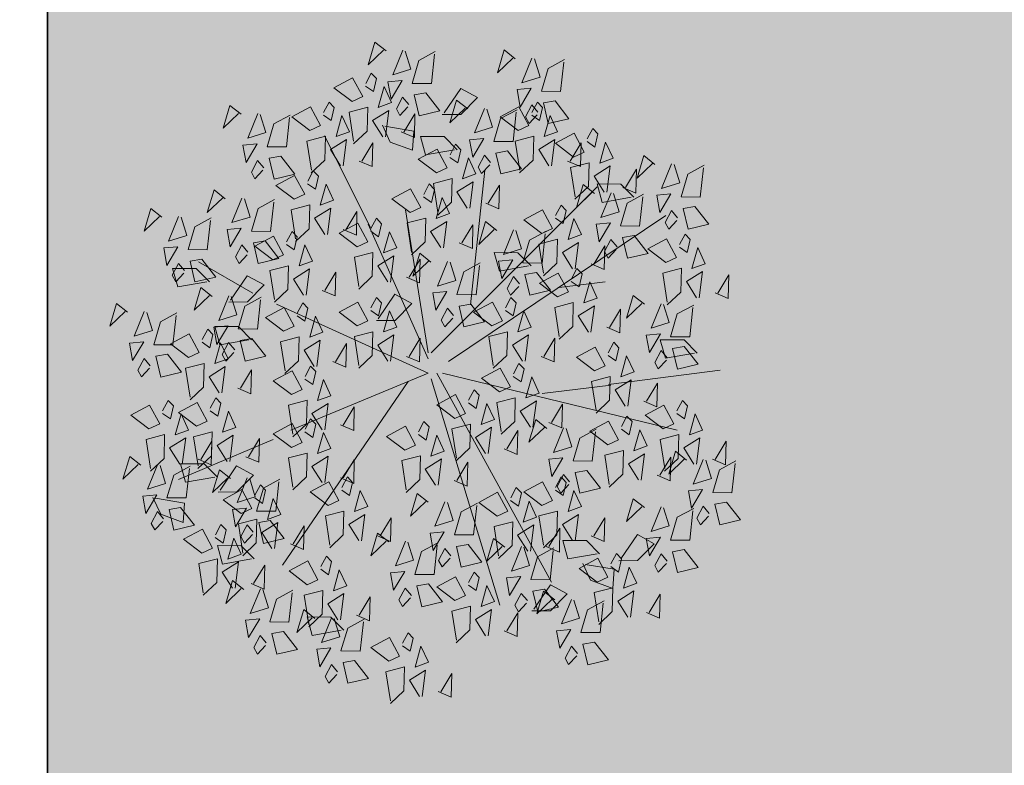
# Model space of a CAD drawing. Units: inches. Extents: x 1704 to 6393, y -157 to 1172.
# Tile 65 of 122: x 1897 to 1937, y 950 to 980. Entities that reach past the tile are written whole.
import ezdxf

# ---------------------------------------------------------------- set-up
doc = ezdxf.new("R2010")
doc.units = ezdxf.units.IN
doc.header["$MEASUREMENT"] = 0
for name, color, linetype, lineweight in [('A-ANNO-DIMS', 7, 'Continuous', 13), ('C-PROP', 7, 'Continuous', 35), ('L-shrub', 74, 'Continuous', 18)]:
    doc.layers.add(name, color=color, linetype=linetype, lineweight=lineweight)
doc.layers.add('L-HRDS-PATT', color=9, linetype='Continuous', lineweight=13, true_color=0xc5c1ba)
doc.styles.get("Standard").update_dxf_attribs({"font": 'arial.ttf'})
doc.dimstyles.get("Standard").update_dxf_attribs({"dimtxt": 6, "dimasz": 2, "dimexe": 0.18, "dimexo": 0.0625, "dimgap": 0.09, "dimtad": 0, "dimtih": 1, "dimtoh": 1, "dimdec": 1, "dimzin": 0, "dimdsep": 46, "dimlunit": 3, "dimtxsty": 'Standard', "dimblk": 'ARCHTICK', "dimcen": 0.09, "dimadec": 0, "dimazin": 0, "dimtfac": 1, "dimtdec": 1, "dimtofl": 0, "dimtmove": 0, "dimatfit": 3, "dimfxl": 1, "dimtolj": 1, "dimtzin": 0, "dimarcsym": 0})

# ---------------------------------------------------------------- blocks, each defined once
blk = doc.blocks.new('flower shrub 2')
at = {"layer": 'L-shrub'}
for p, q in [((-106.23, 211.82), (-92.99, 218)), ((-93.69, 216.06), (-97.6, 193.26)), ((-112.6, 194.32), (-106.23, 211.82)), ((71.95, 198.59), (86.43, 202.67)), ((86.43, 202.67), (86.36, 184.05)), ((-97.6, 193.26), (-112.6, 194.32)), ((-81.12, 192.39), (-66.64, 196.47)), ((-66.64, 196.47), (-66.71, 177.85)), ((75.99, 175.82), (71.95, 198.59)), ((-77.07, 169.62), (-81.12, 192.39)), ((-66.71, 177.85), (-77.08, 167.55)), ((86.36, 184.05), (75.99, 173.75)), ((-145.24, 163.47), (-130.76, 167.54)), ((-141.2, 140.7), (-145.24, 163.47)), ((-130.76, 167.54), (-130.83, 148.93)), ((-88.72, 152.29), (-88.87, 166.9)), ((-87.4, 165.46), (-68.26, 152.47)), ((26.45, 165.53), (40.92, 169.61)), ((30.49, 142.76), (26.45, 165.53)), ((40.92, 169.61), (40.85, 150.99)), ((60.21, 144.02), (60.06, 158.64)), ((61.53, 157.19), (80.67, 144.21)), ((-130.83, 148.93), (-141.21, 138.63)), ((-75.44, 139.25), (-88.72, 152.29)), ((-68.26, 152.47), (-75.44, 139.25)), ((40.85, 150.99), (30.48, 140.69)), ((73.5, 130.99), (60.21, 144.02)), ((80.67, 144.21), (73.5, 130.99)), ((-201.09, 93.22), (-186.61, 97.3)), ((-197.05, 70.45), (-201.09, 93.22)), ((-186.61, 97.3), (-186.68, 78.69)), ((-186.68, 78.69), (-197.06, 68.38)), ((45.73, 28.33), (45.58, 42.95)), ((47.06, 41.5), (66.19, 28.51)), ((179.06, 14.59), (185.43, 32.08)), ((185.43, 32.08), (198.67, 38.26)), ((197.96, 36.32), (194.06, 13.53)), ((59.02, 15.29), (45.73, 28.33)), ((66.19, 28.51), (59.02, 15.29)), ((175.38, 4.39), (189.86, 8.47)), ((194.06, 13.53), (179.06, 14.59)), ((189.86, 8.47), (189.78, -10.15)), ((179.42, -18.38), (175.38, 4.39)), ((189.78, -10.15), (179.41, -20.45)), ((207.07, -23.32), (206.92, -8.7)), ((208.4, -10.15), (227.53, -23.13)), ((227.53, -23.13), (220.36, -36.35)), ((220.36, -36.35), (207.07, -23.32)), ((84.36, -53.46), (98.84, -49.38)), ((88.41, -76.23), (84.36, -53.46)), ((98.84, -49.38), (98.77, -68)), ((98.77, -68), (88.4, -78.3)), ((-181.81, -93.56), (-181.96, -78.94)), ((-180.48, -80.39), (-161.34, -93.38)), ((-168.52, -106.6), (-181.81, -93.56)), ((-161.34, -93.38), (-168.52, -106.6)), ((-141.1, -107.17), (-126.62, -103.09)), ((-137.06, -129.94), (-141.1, -107.17)), ((-126.62, -103.09), (-126.7, -121.71)), ((-157.94, -124.93), (-144.7, -118.75)), ((-145.41, -120.69), (-149.31, -143.48)), ((-126.7, -121.71), (-137.07, -132.01)), ((-164.31, -142.42), (-157.94, -124.93)), ((138.15, -134.03), (152.62, -129.95)), ((152.62, -129.95), (152.55, -148.57)), ((142.19, -156.8), (138.15, -134.03)), ((-149.31, -143.48), (-164.31, -142.42)), ((-142.51, -161.74), (-142.65, -147.12)), ((-141.18, -148.57), (-122.04, -161.55)), ((152.55, -148.57), (142.18, -158.87)), ((-129.22, -174.77), (-142.51, -161.74)), ((-122.04, -161.55), (-129.22, -174.77)), ((16.1, -183.61), (30.58, -179.53)), ((20.14, -206.38), (16.1, -183.61)), ((30.58, -179.53), (30.51, -198.15)), ((30.51, -198.15), (20.14, -208.45))]:
    blk.add_line(p, q, dxfattribs=at)
for points in [[(52.15, 237.83), (59.05, 246.56), (41.2, 251.84), (52.74, 239.81)], [(-67.82, 227.5), (-60.92, 236.23), (-78.77, 241.51), (-67.23, 229.48)], [(-39.32, 221.12), (-28.59, 235.29), (-20.71, 220.61), (-35.41, 212.74), (-39.32, 221.12)], [(29.03, 225.28), (27.99, 236.36), (14.33, 233.94), (29.03, 225.28)], [(52.02, 222.79), (37.77, 218.39), (33.35, 232.62), (52.6, 224.77)], [(-90.95, 214.95), (-91.98, 226.03), (-105.64, 223.61), (-90.95, 214.95)], [(10.23, 220.07), (15.95, 224.84), (6.62, 229.76), (1.48, 226.97), (8.24, 220.66)], [(126.62, 210.97), (133.52, 219.7), (115.67, 224.99), (127.2, 212.95)], [(-109.75, 209.74), (-104.02, 214.51), (-113.35, 219.43), (-118.49, 216.64), (-111.73, 210.33)], [(-67.96, 212.46), (-82.2, 208.06), (-86.62, 222.29), (-67.37, 214.44)], [(-70.39, 219.89), (-47.54, 223.41), (-43.79, 208.84), (-62.4, 209.34), (-72.46, 219.95)], [(49.53, 199.82), (26.54, 202.32), (26.68, 217.36), (44.53, 212.08), (51.52, 199.24)], [(-27.19, 210.46), (-31.5, 204.37), (-21.21, 202.03), (-16.97, 206.05), (-25.13, 210.4)], [(19.2, 206.65), (5.18, 195.71), (1.34, 211.93), (17.57, 215.74), (19.2, 206.65)], [(103.49, 198.43), (102.46, 209.5), (88.8, 207.08), (103.49, 198.43)], [(-100.78, 196.32), (-114.8, 185.38), (-118.63, 201.6), (-102.4, 205.41), (-100.78, 196.32)], [(-70.44, 189.49), (-93.43, 191.99), (-93.29, 207.03), (-75.44, 201.75), (-68.45, 188.91)], [(-66.87, 197.06), (-54.24, 204.99), (-46.3, 192.37), (-66.93, 195)], [(16.53, 190.13), (27.26, 204.31), (35.14, 189.63), (20.44, 181.76), (16.53, 190.13)], [(84.69, 193.22), (90.42, 197.99), (81.09, 202.9), (75.95, 200.11), (82.71, 193.8)], [(126.48, 195.93), (112.24, 191.53), (107.82, 205.76), (127.07, 197.91)], [(-136.54, 179.8), (-125.81, 193.98), (-117.93, 179.3), (-132.63, 171.43), (-136.54, 179.8)], [(-47.57, 123.92), (-79, 197.93)], [(-44.01, 200.58), (-40.16, 190.14), (-27.58, 196), (-44.01, 200.58)], [(-37.25, 183.93), (-26.52, 198.11), (-18.64, 183.43), (-33.34, 175.56), (-37.25, 183.93)], [(-68.32, 182.7), (-45.47, 186.22), (-41.72, 171.65), (-60.33, 172.15), (-70.39, 182.76)], [(-14.54, 188.9), (8.31, 192.42), (12.06, 177.85), (-6.55, 178.35), (-16.61, 188.96)], [(64.56, 171.72), (71.46, 180.45), (53.61, 185.73), (65.15, 173.7)], [(93.66, 179.79), (79.64, 168.86), (75.81, 185.07), (92.04, 188.89), (93.66, 179.79)], [(124, 172.97), (101.01, 175.46), (101.15, 190.5), (119, 185.22), (125.98, 172.38)], [(-167.61, 178.57), (-144.76, 182.09), (-141.01, 167.52), (-159.62, 168.02), (-169.68, 178.63)], [(-63.13, 182.49), (-67.54, 172.28), (-48.93, 171.78), (-63.18, 180.43)], [(28.66, 179.47), (24.35, 173.38), (34.64, 171.04), (38.88, 175.06), (30.72, 179.41)], [(66.94, 139.62), (91.63, 182.23)], [(-78.16, 157.26), (-71.26, 165.99), (-89.12, 171.27), (-77.58, 159.24)], [(-25.12, 173.27), (-29.43, 167.19), (-19.14, 164.84), (-14.9, 168.86), (-23.06, 173.21)], [(-11.02, 166.07), (1.61, 174), (9.54, 161.38), (-11.08, 164.01)], [(41.44, 159.17), (40.4, 170.25), (26.74, 167.83), (41.44, 159.17)], [(141.1, 161.39), (148, 170.12), (130.14, 175.4), (141.68, 163.37)], [(-164.09, 155.74), (-151.46, 163.67), (-143.52, 151.05), (-164.15, 153.68)], [(-124.41, 169.14), (-128.72, 163.05), (-118.43, 160.71), (-114.19, 164.73), (-122.34, 169.08)], [(-105.51, 148.81), (-94.78, 162.99), (-86.9, 148.31), (-101.6, 140.44), (-105.51, 148.81)], [(-64.8, 159.87), (-52.17, 167.8), (-44.24, 155.19), (-64.86, 157.81)], [(-41.95, 163.39), (-38.09, 152.95), (-25.52, 158.81), (-41.95, 163.39)], [(11.84, 169.59), (15.69, 159.15), (28.27, 165.01), (11.84, 169.59)], [(22.64, 153.96), (28.36, 158.73), (19.03, 163.65), (13.89, 160.86), (20.65, 154.55)], [(64.43, 156.68), (50.18, 152.28), (45.76, 166.51), (65.01, 158.66)], [(207.29, 148.99), (214.19, 157.72), (196.34, 163.01), (207.88, 150.97)], [(-165.04, 146.93), (-158.14, 155.66), (-175.99, 160.94), (-164.45, 148.91)], [(-141.23, 159.26), (-137.38, 148.82), (-124.8, 154.68), (-141.23, 159.26)], [(-101.29, 144.71), (-102.33, 155.79), (-115.98, 153.37), (-101.29, 144.71)], [(117.97, 148.84), (116.93, 159.92), (103.28, 157.5), (117.97, 148.84)], [(140.96, 146.35), (126.72, 141.95), (122.3, 156.18), (141.55, 148.33)], [(-136.58, 147.58), (-113.73, 151.1), (-109.98, 136.53), (-128.59, 137.03), (-138.65, 147.64)], [(-120.09, 139.5), (-114.36, 144.27), (-123.69, 149.19), (-128.83, 146.4), (-122.07, 140.09)], [(-78.3, 142.22), (-92.54, 137.81), (-96.96, 152.05), (-77.71, 144.2)], [(-7.28, 151.5), (-11.69, 141.29), (6.92, 140.79), (-7.33, 149.44)], [(31.61, 140.54), (17.59, 129.6), (13.76, 145.82), (29.99, 149.63), (31.61, 140.54)], [(61.95, 133.71), (38.95, 136.21), (39.09, 151.25), (56.94, 145.97), (63.93, 133.13)], [(99.17, 143.63), (104.9, 148.4), (95.57, 153.32), (90.43, 150.53), (97.19, 144.22)], [(184.16, 136.45), (183.13, 147.53), (169.47, 145.1), (184.16, 136.45)], [(-188.17, 134.38), (-189.2, 145.46), (-202.86, 143.04), (-188.17, 134.38)], [(-165.18, 131.89), (-179.42, 127.48), (-183.84, 141.72), (-164.59, 133.87)], [(-160.34, 141.17), (-164.76, 130.96), (-146.15, 130.46), (-160.4, 139.11)], [(-61.06, 145.31), (-65.47, 135.09), (-46.86, 134.59), (-61.11, 143.24)], [(108.14, 130.21), (94.12, 119.27), (90.29, 135.49), (106.52, 139.3), (108.14, 130.21)], [(138.48, 123.38), (115.49, 125.88), (115.63, 140.92), (133.48, 135.64), (140.46, 122.8)], [(165.36, 131.24), (171.09, 136.01), (161.76, 140.92), (156.62, 138.13), (163.38, 131.82)], [(207.15, 133.95), (192.91, 129.55), (188.49, 143.78), (207.74, 135.93)], [(-206.97, 129.17), (-201.24, 133.94), (-210.57, 138.86), (-215.71, 136.07), (-208.95, 129.76)], [(-133.06, 124.75), (-120.43, 132.68), (-112.5, 120.06), (-133.12, 122.69)], [(-111.12, 126.07), (-125.14, 115.14), (-128.97, 131.36), (-112.74, 135.17), (-111.12, 126.07)], [(-80.78, 119.25), (-103.77, 121.75), (-103.63, 136.79), (-85.78, 131.5), (-78.8, 118.66)], [(-93.39, 138.15), (-97.69, 132.06), (-87.4, 129.72), (-83.16, 133.74), (-91.32, 138.09)], [(93.06, 124.02), (103.79, 138.2), (111.67, 123.52), (96.98, 115.65), (93.06, 124.02)], [(-198, 115.75), (-212.02, 104.81), (-215.85, 121.03), (-199.62, 124.84), (-198, 115.75)], [(-167.66, 108.92), (-190.65, 111.42), (-190.51, 126.46), (-172.66, 121.17), (-165.67, 108.33)], [(-110.21, 128.27), (-106.35, 117.83), (-93.78, 123.69), (-110.21, 128.27)], [(-53.8, 109.56), (-43.07, 123.73), (-35.19, 109.05), (-49.89, 101.18), (-53.8, 109.56)], [(-12.43, 109.56), (-1.7, 123.73), (6.18, 109.05), (-8.52, 101.18), (-12.43, 109.56)], [(37.21, 115.75), (47.94, 129.93), (55.82, 115.25), (41.13, 107.38), (37.21, 115.75)], [(61.99, 122.79), (84.85, 126.31), (88.59, 111.74), (69.98, 112.24), (59.92, 122.85)], [(174.33, 117.81), (160.31, 106.88), (156.48, 123.09), (172.71, 126.91), (174.33, 117.81)], [(204.67, 110.99), (181.68, 113.48), (181.82, 128.52), (199.67, 123.24), (206.65, 110.4)], [(-2.25, 17.94), (-145.94, 116.61)], [(6.14, 114.53), (29, 118.04), (32.74, 103.47), (14.13, 103.98), (4.07, 114.58)], [(4.49, 2.24), (58.38, 121.09)], [(140.64, 107.49), (151.37, 121.67), (159.25, 106.99), (144.55, 99.12), (140.64, 107.49)], [(-161.36, 97.16), (-150.63, 111.34), (-142.75, 96.66), (-157.45, 88.79), (-161.36, 97.16)], [(-129.32, 110.18), (-133.73, 99.97), (-115.12, 99.47), (-129.37, 108.12)], [(-84.87, 108.33), (-62.02, 111.85), (-58.27, 97.28), (-76.88, 97.78), (-86.94, 108.38)], [(-43.5, 108.33), (-20.65, 111.85), (-16.9, 97.28), (-35.51, 97.78), (-45.57, 108.38)], [(4.49, 2.24), (-40.41, 109.88)], [(105.19, 113.36), (100.89, 107.27), (111.17, 104.93), (115.42, 108.95), (107.26, 113.3)], [(109.57, 106.26), (132.42, 109.78), (136.17, 95.21), (117.56, 95.71), (107.5, 106.32)], [(194.42, 95.09), (205.15, 109.27), (213.03, 94.59), (198.33, 86.72), (194.42, 95.09)], [(-187.79, 91.15), (-180.89, 99.88), (-198.75, 105.16), (-187.21, 93.13)], [(49.34, 105.09), (45.04, 99.01), (55.32, 96.67), (59.57, 100.68), (51.41, 105.04)], [(65.51, 99.96), (78.14, 107.89), (86.08, 95.27), (65.46, 97.9)], [(88.37, 103.48), (92.23, 93.04), (104.8, 98.9), (88.37, 103.48)], [(-192.43, 95.93), (-169.58, 99.45), (-165.83, 84.88), (-184.44, 85.38), (-194.5, 95.99)], [(-99.31, 80.63), (-88.58, 94.81), (-80.7, 80.13), (-95.39, 72.26), (-99.31, 80.63)], [(-81.35, 85.5), (-68.72, 93.43), (-60.78, 80.81), (-81.41, 83.43)], [(-41.67, 98.9), (-45.98, 92.81), (-35.69, 90.47), (-31.45, 94.49), (-39.6, 98.84)], [(-39.98, 85.5), (-27.35, 93.43), (-19.41, 80.81), (-40.04, 83.43)], [(-0.3, 98.9), (-4.61, 92.81), (5.68, 90.47), (9.92, 94.49), (1.76, 98.84)], [(9.66, 91.7), (22.29, 99.62), (30.23, 87.01), (9.61, 89.63)], [(32.52, 95.21), (36.38, 84.78), (48.95, 90.64), (32.52, 95.21)], [(152.77, 96.83), (148.46, 90.75), (158.75, 88.4), (162.99, 92.42), (154.83, 96.77)], [(163.35, 93.87), (186.2, 97.38), (189.95, 82.82), (171.34, 83.32), (161.28, 93.92)], [(-210.92, 78.6), (-211.96, 89.68), (-225.62, 87.26), (-210.92, 78.6)], [(-187.93, 76.11), (-202.17, 71.7), (-206.59, 85.94), (-187.34, 78.09)], [(-149.23, 86.5), (-153.54, 80.42), (-143.25, 78.07), (-139.01, 82.09), (-147.17, 86.44)], [(-58.49, 89.02), (-54.64, 78.58), (-42.06, 84.44), (-58.49, 89.02)], [(-17.12, 89.02), (-13.27, 78.58), (-0.69, 84.44), (-17.12, 89.02)], [(69.26, 85.39), (64.84, 75.18), (83.45, 74.68), (69.2, 83.33)], [(113.09, 83.43), (125.72, 91.36), (133.65, 78.75), (113.03, 81.37)], [(135.94, 86.95), (139.8, 76.51), (152.38, 82.37), (135.94, 86.95)], [(-229.72, 73.39), (-223.99, 78.16), (-233.32, 83.08), (-238.46, 80.29), (-231.7, 73.98)], [(-188.91, 73.1), (-176.28, 81.03), (-168.35, 68.42), (-188.97, 71.04)], [(-130.38, 79.41), (-107.52, 82.92), (-103.78, 68.35), (-122.39, 68.86), (-132.45, 79.46)], [(118.58, 47.68), (190.43, 83.56)], [(166.87, 71.04), (179.5, 78.96), (187.44, 66.35), (166.81, 68.97)], [(206.55, 84.43), (202.24, 78.35), (212.53, 76.01), (216.77, 80.02), (208.61, 84.38)], [(-190.41, 53.14), (-213.4, 55.64), (-213.26, 70.68), (-195.41, 65.39), (-188.43, 52.55)], [(-166.05, 76.62), (-162.2, 66.18), (-149.62, 72.04), (-166.05, 76.62)], [(-87.18, 69.97), (-91.48, 63.89), (-81.2, 61.54), (-76.95, 65.56), (-85.11, 69.92)], [(-77.6, 70.93), (-82.02, 60.72), (-63.41, 60.22), (-77.66, 68.87)], [(-36.23, 70.93), (-40.65, 60.72), (-22.04, 60.22), (-36.29, 68.87)], [(13.41, 77.13), (8.99, 66.92), (27.6, 66.41), (13.35, 75.06)], [(41.35, 57.91), (52.08, 72.09), (59.96, 57.41), (45.26, 49.54), (41.35, 57.91)], [(103.41, 57.91), (114.13, 72.09), (122.01, 57.41), (107.32, 49.54), (103.41, 57.91)], [(189.73, 74.55), (193.58, 64.12), (206.16, 69.98), (189.73, 74.55)], [(217.17, 62.04), (227.9, 76.22), (235.78, 61.54), (221.08, 53.67), (217.17, 62.04)], [(-220.75, 59.96), (-234.77, 49.03), (-238.6, 65.25), (-222.37, 69.06), (-220.75, 59.96)], [(-126.86, 56.58), (-114.23, 64.5), (-106.29, 51.89), (-126.91, 54.51)], [(116.83, 68.87), (112.42, 58.65), (131.03, 58.15), (116.78, 66.8)], [(186.1, 60.81), (208.96, 64.33), (212.7, 49.76), (194.09, 50.26), (184.03, 60.87)], [(-185.17, 58.54), (-189.58, 48.32), (-170.97, 47.82), (-185.22, 56.47)], [(-104, 60.09), (-100.14, 49.66), (-87.57, 55.52), (-104, 60.09)], [(10.28, 56.68), (33.14, 60.2), (36.88, 45.63), (18.27, 46.13), (8.21, 56.74)], [(72.33, 56.68), (95.19, 60.2), (98.94, 45.63), (80.33, 46.13), (70.27, 56.74)], [(170.61, 56.47), (166.2, 46.26), (184.81, 45.75), (170.56, 54.41)], [(-221.35, 33.12), (-210.62, 47.29), (-202.74, 32.61), (-217.44, 24.74), (-221.35, 33.12)], [(-127.81, 33.3), (-120.91, 42.03), (-138.76, 47.31), (-127.22, 35.28)], [(15.72, 2.24), (121.24, 49.33)], [(53.48, 47.25), (49.18, 41.16), (59.46, 38.82), (63.71, 42.84), (55.55, 47.19)], [(115.53, 47.25), (111.23, 41.16), (121.51, 38.82), (125.76, 42.84), (117.6, 47.19)], [(229.3, 51.38), (225, 45.3), (235.28, 42.95), (239.53, 46.97), (231.37, 51.32)], [(256.93, 35.37), (263.83, 44.1), (245.98, 49.38), (257.52, 37.35)], [(-123.11, 42.01), (-127.53, 31.79), (-108.92, 31.29), (-123.17, 39.94)], [(13.8, 33.85), (26.43, 41.78), (34.37, 29.16), (13.74, 31.79)], [(75.86, 33.85), (88.48, 41.78), (96.42, 29.16), (75.8, 31.79)], [(189.62, 37.98), (202.25, 45.91), (210.19, 33.29), (189.57, 35.92)], [(212.48, 41.5), (216.34, 31.06), (228.91, 36.92), (212.48, 41.5)], [(-252.42, 31.89), (-229.56, 35.41), (-225.82, 20.84), (-244.43, 21.34), (-254.49, 31.94)], [(-150.93, 20.75), (-151.97, 31.83), (-165.63, 29.41), (-150.93, 20.75)], [(-55.87, 20.72), (-45.14, 34.9), (-37.26, 20.22), (-51.96, 12.35), (-55.87, 20.72)], [(36.66, 37.37), (40.51, 26.93), (53.09, 32.79), (36.66, 37.37)], [(98.71, 37.37), (102.57, 26.93), (115.14, 32.79), (98.71, 37.37)], [(233.81, 22.82), (232.77, 33.9), (219.11, 31.48), (233.81, 22.82)], [(-169.73, 15.55), (-164.01, 20.31), (-173.34, 25.23), (-178.48, 22.44), (-171.72, 16.13)], [(-127.94, 18.26), (-142.19, 13.86), (-146.61, 28.09), (-127.36, 20.24)], [(130.3, 16.59), (141.02, 30.77), (148.91, 16.09), (134.21, 8.22), (130.3, 16.59)], [(193.37, 23.42), (188.95, 13.2), (207.56, 12.7), (193.31, 21.35)], [(215.01, 17.61), (220.73, 22.38), (211.4, 27.3), (206.26, 24.51), (213.02, 18.2)], [(256.8, 20.33), (242.55, 15.92), (238.13, 30.16), (257.38, 22.31)], [(-248.9, 9.06), (-236.27, 16.99), (-228.33, 4.37), (-248.95, 7)], [(-209.22, 22.46), (-213.52, 16.37), (-203.24, 14.03), (-198.99, 18.05), (-207.15, 22.4)], [(-96.78, 2.31), (-89.88, 11.04), (-107.73, 16.33), (-96.19, 4.29)], [(-86.94, 19.49), (-64.08, 23.01), (-60.34, 8.44), (-78.95, 8.94), (-89.01, 19.55)], [(17.55, 19.28), (13.13, 9.07), (31.74, 8.57), (17.49, 17.22)], [(20.21, 2.24), (132.47, 20.18)], [(79.6, 19.28), (75.19, 9.07), (93.8, 8.57), (79.54, 17.22)], [(99.22, 15.36), (122.08, 18.88), (125.83, 4.31), (107.22, 4.81), (97.16, 15.42)], [(-226.04, 12.58), (-222.18, 2.14), (-209.61, 8), (-226.04, 12.58)], [(-160.76, 2.12), (-174.78, -8.81), (-178.61, 7.4), (-162.38, 11.22), (-160.76, 2.12)], [(-130.42, -4.7), (-153.42, -2.21), (-153.28, 12.83), (-135.43, 7.55), (-128.44, -5.29)], [(-43.74, 10.06), (-48.04, 3.98), (-37.76, 1.63), (-33.51, 5.65), (-41.67, 10)], [(91.45, 0.25), (98.35, 8.98), (80.5, 14.26), (92.04, 2.23)], [(161.32, -4.07), (172.05, 10.11), (179.93, -4.57), (165.24, -12.44), (161.32, -4.07)], [(223.98, 4.18), (209.96, -6.75), (206.13, 9.47), (222.35, 13.28), (223.98, 4.18)], [(254.32, -2.64), (231.32, -0.14), (231.46, 14.9), (249.31, 9.61), (256.3, -3.23)], [(0, 0), (-177.37, -53.82)], [(-119.91, -10.23), (-120.94, 0.84), (-134.6, -1.58), (-119.91, -10.23)], [(-83.42, -3.34), (-70.79, 4.59), (-62.85, -8.02), (-83.47, -5.4)], [(-60.56, 0.18), (-56.71, -10.26), (-44.13, -4.4), (-60.56, 0.18)], [(20.21, 0), (150.43, -130.06)], [(102.75, -7.47), (115.38, 0.46), (123.31, -12.16), (102.69, -9.53)], [(142.42, 5.93), (138.12, -0.16), (148.4, -2.5), (152.65, 1.52), (144.49, 5.87)], [(-245.15, -5.51), (-249.57, -15.72), (-230.96, -16.22), (-245.21, -7.57)], [(-173.77, -18.53), (-163.04, -4.35), (-155.16, -19.03), (-169.86, -26.9), (-173.77, -18.53)], [(4.49, -4.48), (-159.41, -94.18)], [(-138.71, -15.44), (-132.98, -10.67), (-142.31, -5.76), (-147.45, -8.55), (-140.69, -14.86)], [(-96.92, -12.73), (-111.16, -17.13), (-115.58, -2.9), (-96.33, -10.75)], [(-31.05, -18.53), (-20.32, -4.35), (-12.44, -19.03), (-27.13, -26.9), (-31.05, -18.53)], [(68.33, -12.3), (67.29, -1.22), (53.63, -3.64), (68.33, -12.3)], [(91.32, -14.79), (77.07, -19.2), (72.66, -4.96), (91.9, -12.81)], [(125.6, -3.95), (129.46, -14.39), (142.03, -8.53), (125.6, -3.95)], [(130.25, -5.3), (153.11, -1.78), (156.85, -16.35), (138.24, -15.85), (128.18, -5.24)], [(4.49, -8.97), (-40.41, -192.85)], [(13.47, -13.45), (127.98, -183.88)], [(49.53, -17.51), (55.25, -12.74), (45.92, -7.82), (40.78, -10.61), (47.54, -16.92)], [(173.45, -14.73), (169.15, -20.81), (179.43, -23.16), (183.68, -19.14), (175.52, -14.79)], [(211.43, -28.68), (218.32, -19.95), (200.47, -14.66), (212.01, -26.7)], [(-204.84, -19.76), (-181.99, -16.24), (-178.24, -30.81), (-196.85, -30.31), (-206.91, -19.7)], [(-129.74, -28.87), (-143.76, -39.8), (-147.59, -23.59), (-131.36, -19.77), (-129.74, -28.87)], [(-99.4, -35.69), (-122.39, -33.2), (-122.25, -18.16), (-104.4, -23.44), (-97.41, -36.28)], [(-79.67, -17.9), (-84.09, -28.12), (-65.48, -28.62), (-79.73, -19.97)], [(-62.12, -19.76), (-39.26, -16.24), (-35.52, -30.81), (-54.13, -30.31), (-64.19, -19.7)], [(58.5, -30.94), (44.48, -41.87), (40.65, -25.65), (56.88, -21.84), (58.5, -30.94)], [(88.84, -37.76), (65.84, -35.27), (65.98, -20.22), (83.83, -25.51), (90.82, -38.35)], [(106.49, -22.04), (102.08, -32.25), (120.69, -32.75), (106.44, -24.1)], [(133.77, -28.13), (146.4, -20.2), (154.34, -32.82), (133.72, -30.19)], [(-161.65, -29.19), (-165.95, -35.28), (-155.67, -37.62), (-151.42, -33.6), (-159.58, -29.25)], [(-18.92, -29.19), (-23.22, -35.28), (-12.94, -37.62), (-8.69, -33.6), (-16.85, -29.25)], [(57.96, -30.81), (163.48, -42.02)], [(156.63, -24.61), (160.49, -35.05), (173.06, -29.19), (156.63, -24.61)], [(188.3, -41.22), (187.26, -30.14), (173.6, -32.57), (188.3, -41.22)], [(-201.32, -42.59), (-188.69, -34.66), (-180.76, -47.28), (-201.38, -44.65)], [(-107.58, -51.59), (-96.85, -37.41), (-88.97, -52.09), (-103.67, -59.96), (-107.58, -51.59)], [(-58.6, -42.59), (-45.97, -34.66), (-38.03, -47.28), (-58.65, -44.65)], [(41.35, -47.45), (52.08, -33.28), (59.96, -47.96), (45.26, -55.83), (41.35, -47.45)], [(116.28, -51.4), (123.17, -42.67), (105.32, -37.39), (116.86, -49.42)], [(169.5, -46.43), (175.23, -41.66), (165.89, -36.75), (160.76, -39.54), (167.52, -45.85)], [(211.29, -43.72), (197.04, -48.12), (192.63, -33.89), (211.88, -41.74)], [(-178.47, -39.07), (-174.61, -49.51), (-162.04, -43.65), (-178.47, -39.07)], [(-131.94, -57.6), (-125.04, -48.87), (-142.9, -43.59), (-131.36, -55.62)], [(-35.74, -39.07), (-31.88, -49.51), (-19.31, -43.65), (-35.74, -39.07)], [(-10.36, -53.65), (0.37, -39.48), (8.25, -54.15), (-6.45, -62.02), (-10.36, -53.65)], [(10.28, -48.68), (33.14, -45.17), (36.88, -59.73), (18.27, -59.23), (8.21, -48.63)], [(137.52, -42.69), (133.1, -52.91), (151.71, -53.41), (137.46, -44.76)], [(-138.65, -52.81), (-115.8, -49.3), (-112.05, -63.87), (-130.66, -63.36), (-140.72, -52.76)], [(-41.43, -54.88), (-18.58, -51.36), (-14.83, -65.93), (-33.44, -65.43), (-43.5, -54.82)], [(93.15, -63.95), (92.11, -52.87), (78.45, -55.29), (93.15, -63.95)], [(178.47, -59.86), (164.45, -70.79), (160.62, -54.58), (176.85, -50.76), (178.47, -59.86)], [(208.81, -66.68), (185.82, -64.19), (185.95, -49.15), (203.81, -54.43), (210.79, -67.27)], [(194.42, -68.11), (205.15, -53.94), (213.03, -68.62), (198.33, -76.49), (194.42, -68.11)], [(250.73, -65.86), (257.63, -57.13), (239.78, -51.85), (251.31, -63.88)], [(-197.58, -57.16), (-201.99, -67.37), (-183.38, -67.87), (-197.63, -59.22)], [(-155.07, -70.15), (-156.11, -59.07), (-169.77, -61.49), (-155.07, -70.15)], [(-54.85, -57.16), (-59.27, -67.37), (-40.66, -67.87), (-54.91, -59.22)], [(53.48, -58.12), (49.18, -64.2), (59.46, -66.54), (63.71, -62.52), (55.55, -58.17)], [(74.35, -69.16), (80.08, -64.39), (70.74, -59.47), (65.6, -62.26), (72.37, -68.57)], [(116.14, -66.44), (101.89, -70.85), (97.48, -56.61), (116.73, -64.46)], [(-173.87, -75.36), (-168.14, -70.59), (-177.47, -65.67), (-182.61, -68.46), (-175.85, -74.77)], [(-132.08, -72.64), (-146.33, -77.04), (-150.74, -62.81), (-131.49, -70.66)], [(-135.13, -75.64), (-122.5, -67.72), (-114.56, -80.33), (-135.19, -77.71)], [(-95.45, -62.25), (-99.76, -68.33), (-89.47, -70.68), (-85.23, -66.66), (-93.39, -62.3)], [(1.77, -64.31), (-2.54, -70.4), (7.75, -72.74), (11.99, -68.72), (3.83, -64.37)], [(13.8, -71.51), (26.43, -63.59), (34.37, -76.2), (13.74, -73.58)], [(36.66, -67.99), (40.51, -78.43), (53.09, -72.57), (36.66, -67.99)], [(163.35, -69.34), (186.2, -65.83), (189.95, -80.39), (171.34, -79.89), (161.28, -69.29)], [(227.6, -78.41), (226.56, -67.33), (212.91, -69.75), (227.6, -78.41)], [(-112.27, -72.13), (-108.42, -82.56), (-95.84, -76.7), (-112.27, -72.13)], [(-99.31, -86.71), (-88.58, -72.53), (-80.7, -87.21), (-95.39, -95.08), (-99.31, -86.71)], [(-38.86, -90.66), (-31.96, -81.92), (-49.81, -76.64), (-38.27, -88.67)], [(-37.91, -77.71), (-25.28, -69.78), (-17.35, -82.4), (-37.97, -79.77)], [(-15.06, -74.19), (-11.2, -84.63), (1.38, -78.77), (-15.06, -74.19)], [(83.32, -82.58), (69.3, -93.52), (65.47, -77.3), (81.7, -73.49), (83.32, -82.58)], [(113.66, -89.41), (90.67, -86.91), (90.8, -71.87), (108.65, -77.16), (115.64, -90)], [(113.75, -86.71), (124.48, -72.53), (132.36, -87.21), (117.66, -95.08), (113.75, -86.71)], [(208.8, -83.62), (214.53, -78.85), (205.2, -73.93), (200.06, -76.72), (206.82, -83.03)], [(250.59, -80.9), (236.35, -85.31), (231.93, -71.07), (251.18, -78.92)], [(-173.31, -96.85), (-166.41, -88.12), (-184.27, -82.84), (-172.73, -94.87)], [(-164.9, -88.78), (-178.92, -99.72), (-182.75, -83.5), (-166.52, -79.68), (-164.9, -88.78)], [(-134.56, -95.61), (-157.55, -93.11), (-157.42, -78.07), (-139.56, -83.35), (-132.58, -96.19)], [(-130.38, -87.94), (-107.52, -84.42), (-103.78, -98.99), (-122.39, -98.48), (-132.45, -87.88)], [(82.68, -87.94), (105.53, -84.42), (109.28, -98.99), (90.67, -98.48), (80.61, -87.88)], [(166.87, -92.17), (179.5, -84.24), (187.44, -96.86), (166.81, -94.24)], [(206.55, -78.77), (202.24, -84.86), (212.53, -87.2), (216.77, -83.18), (208.61, -78.83)], [(-131.39, -90.21), (-135.8, -100.43), (-117.19, -100.93), (-131.44, -92.28)], [(-61.99, -103.2), (-63.02, -92.12), (-76.68, -94.54), (-61.99, -103.2)], [(-34.17, -92.28), (-38.58, -102.49), (-19.97, -102.99), (-34.22, -94.34)], [(-4.91, -140.69), (-11.65, -86.87)], [(17.55, -86.08), (13.13, -96.29), (31.74, -96.8), (17.49, -88.14)], [(64.1, -99.1), (74.83, -84.93), (82.71, -99.61), (68.02, -107.48), (64.1, -99.1)], [(189.73, -88.65), (193.58, -99.09), (206.16, -93.23), (189.73, -88.65)], [(217.77, -97.05), (203.75, -107.98), (199.92, -91.76), (216.15, -87.95), (217.77, -97.05)], [(248.11, -103.87), (225.12, -101.38), (225.26, -86.33), (243.11, -91.62), (250.09, -104.46)], [(-196.44, -109.4), (-197.48, -98.32), (-211.14, -100.74), (-196.44, -109.4)], [(-87.18, -97.37), (-91.48, -103.45), (-81.2, -105.8), (-76.95, -101.78), (-85.11, -97.42)], [(-80.79, -108.41), (-75.06, -103.64), (-84.39, -98.73), (-89.53, -101.51), (-82.77, -107.82)], [(-39, -105.7), (-53.24, -110.1), (-57.66, -95.86), (-38.41, -103.72)], [(33.03, -100.33), (55.89, -96.81), (59.63, -111.38), (41.02, -110.88), (30.96, -100.28)], [(125.88, -97.37), (121.57, -103.45), (131.86, -105.8), (136.1, -101.78), (127.94, -97.42)], [(173.73, -111.5), (184.46, -97.32), (192.34, -112), (177.65, -119.87), (173.73, -111.5)], [(-215.24, -114.61), (-209.51, -109.84), (-218.84, -104.92), (-223.98, -107.71), (-217.22, -114.02)], [(-173.45, -111.89), (-187.7, -116.3), (-192.11, -102.06), (-172.86, -109.91)], [(-126.86, -110.76), (-114.23, -102.84), (-106.29, -115.45), (-126.91, -112.83)], [(-104, -107.25), (-100.14, -117.69), (-87.57, -111.82), (-104, -107.25)], [(71.43, -100.32), (75.92, -136.2)], [(86.2, -110.76), (98.83, -102.84), (106.76, -115.45), (86.14, -112.83)], [(109.05, -107.25), (112.91, -117.69), (125.48, -111.82), (109.05, -107.25)], [(170.61, -106.74), (166.2, -116.95), (184.81, -117.46), (170.56, -108.8)], [(-71.82, -121.84), (-85.84, -132.77), (-89.67, -116.56), (-73.44, -112.74), (-71.82, -121.84)], [(-41.48, -128.66), (-64.47, -126.17), (-64.33, -111.13), (-46.48, -116.41), (-39.5, -129.25)], [(6.19, -128.03), (16.91, -113.85), (24.8, -128.53), (10.1, -136.4), (6.19, -128.03)], [(36.55, -123.16), (49.18, -115.23), (57.12, -127.85), (36.5, -125.22)], [(76.23, -109.76), (71.93, -115.85), (82.21, -118.19), (86.46, -114.17), (78.3, -109.82)], [(145.23, -127.84), (152.13, -119.11), (134.28, -113.83), (145.82, -125.86)], [(142.66, -112.73), (165.52, -109.21), (169.26, -123.78), (150.65, -123.28), (140.59, -112.67)], [(-206.27, -128.04), (-220.29, -138.97), (-224.12, -122.75), (-207.89, -118.94), (-206.27, -128.04)], [(-175.93, -134.86), (-198.92, -132.36), (-198.79, -117.32), (-180.93, -122.61), (-173.95, -135.45)], [(-159.29, -130.09), (-148.56, -115.91), (-140.68, -130.59), (-155.38, -138.46), (-159.29, -130.09)], [(59.41, -119.64), (63.27, -130.08), (75.84, -124.22), (59.41, -119.64)], [(185.86, -122.16), (181.56, -128.24), (191.84, -130.59), (196.09, -126.57), (187.93, -122.22)], [(-190.37, -131.32), (-167.51, -127.8), (-163.76, -142.37), (-182.37, -141.87), (-192.43, -131.26)], [(-123.11, -125.33), (-127.53, -135.55), (-108.92, -136.05), (-123.17, -127.4)], [(-51.73, -138.36), (-41, -124.18), (-33.12, -138.86), (-47.82, -146.73), (-51.73, -138.36)], [(-24.89, -129.25), (-2.03, -125.74), (1.72, -140.31), (-16.89, -139.8), (-26.95, -129.2)], [(89.94, -125.33), (85.53, -135.55), (104.14, -136.05), (89.89, -127.4)], [(122.11, -140.39), (121.07, -129.31), (107.41, -131.73), (122.11, -140.39)], [(146.18, -135.56), (158.81, -127.63), (166.75, -140.24), (146.13, -137.62)], [(-82.8, -139.58), (-59.95, -136.07), (-56.2, -150.64), (-74.81, -150.13), (-84.87, -139.53)], [(18.31, -138.69), (14.01, -144.77), (24.29, -147.12), (28.54, -143.1), (20.38, -138.74)], [(40.3, -137.73), (35.89, -147.94), (54.49, -148.44), (40.24, -139.79)], [(103.31, -145.6), (109.03, -140.83), (99.7, -135.91), (94.56, -138.7), (101.33, -145.01)], [(145.1, -142.88), (130.85, -147.29), (126.44, -133.05), (145.68, -140.9)], [(169.04, -132.04), (172.9, -142.48), (185.47, -136.62), (169.04, -132.04)], [(-186.84, -154.15), (-174.21, -146.22), (-166.28, -158.84), (-186.9, -156.21)], [(-147.17, -140.75), (-151.47, -146.84), (-141.19, -149.18), (-136.94, -145.16), (-145.1, -140.81)], [(-21.36, -152.08), (-8.73, -144.16), (-0.8, -156.77), (-21.42, -154.15)], [(-4.49, -139.03), (6.74, -226.49)], [(-163.99, -150.63), (-160.13, -161.07), (-147.56, -155.21), (-163.99, -150.63)], [(-100.92, -167.09), (-94.02, -158.36), (-111.87, -153.08), (-100.33, -165.11)], [(-39.6, -149.02), (-43.91, -155.1), (-33.62, -157.44), (-29.38, -153.43), (-37.54, -149.07)], [(1.49, -148.57), (5.35, -159), (17.92, -153.14), (1.49, -148.57)], [(58.36, -167.09), (65.26, -158.36), (47.41, -153.08), (58.94, -165.11)], [(112.28, -159.02), (98.26, -169.96), (94.43, -153.74), (110.66, -149.93), (112.28, -159.02)], [(142.62, -165.85), (119.63, -163.35), (119.76, -148.31), (137.61, -153.6), (144.6, -166.44)], [(149.93, -150.12), (145.52, -160.34), (164.12, -160.84), (149.87, -152.19)], [(-79.28, -162.41), (-66.65, -154.49), (-58.72, -167.1), (-79.34, -164.48)], [(-56.42, -158.9), (-52.57, -169.33), (-39.99, -163.47), (-56.42, -158.9)], [(167.99, -175.36), (174.89, -166.63), (157.04, -161.34), (168.57, -173.38)], [(-183.1, -168.72), (-187.51, -178.93), (-168.9, -179.43), (-183.15, -170.78)], [(-124.04, -179.64), (-125.08, -168.56), (-138.74, -170.98), (-124.04, -179.64)], [(-39.32, -181.74), (-28.59, -167.56), (-20.71, -182.24), (-35.41, -190.11), (-39.32, -181.74)], [(-17.62, -166.65), (-22.03, -176.87), (-3.42, -177.37), (-17.67, -168.72)], [(35.23, -179.64), (34.2, -168.56), (20.54, -170.98), (35.23, -179.64)], [(90.99, -183.81), (101.72, -169.63), (109.6, -184.31), (94.91, -192.18), (90.99, -183.81)], [(-142.84, -184.85), (-137.12, -180.08), (-146.45, -175.17), (-151.59, -177.95), (-144.83, -184.26)], [(-101.05, -182.14), (-115.3, -186.54), (-119.71, -172.3), (-100.47, -180.15)], [(-75.54, -176.98), (-79.95, -187.19), (-61.34, -187.7), (-75.59, -179.05)], [(16.43, -184.85), (22.16, -180.08), (12.83, -175.17), (7.69, -177.95), (14.45, -184.26)], [(58.22, -182.14), (43.98, -186.54), (39.56, -172.3), (58.81, -180.15)], [(144.86, -187.9), (143.83, -176.83), (130.17, -179.25), (144.86, -187.9)], [(-70.39, -182.97), (-47.54, -179.45), (-43.79, -194.02), (-62.4, -193.52), (-72.46, -182.91)], [(59.92, -185.03), (82.78, -181.52), (86.52, -196.09), (67.91, -195.58), (57.85, -184.98)], [(126.06, -193.11), (131.79, -188.35), (122.46, -183.43), (117.32, -186.22), (124.08, -192.53)], [(167.85, -190.4), (153.61, -194.8), (149.19, -180.57), (168.44, -188.42)], [(-133.87, -198.28), (-147.89, -209.21), (-151.72, -192.99), (-135.49, -189.18), (-133.87, -198.28)], [(-103.53, -205.1), (-126.52, -202.61), (-126.39, -187.57), (-108.54, -192.85), (-101.55, -205.69)], [(-63.68, -200.15), (-56.78, -191.42), (-74.64, -186.14), (-63.1, -198.17)], [(-27.19, -192.4), (-31.5, -198.49), (-21.21, -200.83), (-16.97, -196.81), (-25.13, -192.46)], [(25.4, -198.28), (11.38, -209.21), (7.55, -192.99), (23.78, -189.18), (25.4, -198.28)], [(55.74, -205.1), (32.75, -202.61), (32.89, -187.57), (50.74, -192.85), (57.72, -205.69)], [(-66.87, -205.8), (-54.24, -197.87), (-46.3, -210.49), (-66.93, -207.86)], [(63.44, -207.86), (76.07, -199.94), (84.01, -212.55), (63.39, -209.93)], [(103.12, -194.47), (98.82, -200.55), (109.1, -202.9), (113.35, -198.88), (105.19, -194.52)], [(135.03, -206.54), (121.01, -217.47), (117.18, -201.26), (133.41, -197.44), (135.03, -206.54)], [(165.37, -213.36), (142.38, -210.87), (142.52, -195.83), (160.37, -201.11), (167.35, -213.95)], [(-105.61, -217.91), (-99.88, -213.14), (-109.21, -208.22), (-114.35, -211.01), (-107.59, -217.32)], [(-86.81, -212.7), (-87.85, -201.62), (-101.51, -204.04), (-86.81, -212.7)], [(-63.82, -215.19), (-78.07, -219.59), (-82.48, -205.36), (-63.23, -213.21)], [(-44.01, -202.28), (-40.16, -212.72), (-27.58, -206.86), (-44.01, -202.28)], [(86.3, -204.35), (90.16, -214.78), (102.73, -208.92), (86.3, -204.35)], [(-96.64, -231.33), (-110.66, -242.26), (-114.49, -226.05), (-98.26, -222.23), (-96.64, -231.33)], [(-66.3, -238.16), (-89.29, -235.66), (-89.16, -220.62), (-71.3, -225.9), (-64.32, -238.74)], [(-63.13, -220.37), (-67.54, -230.58), (-48.93, -231.08), (-63.18, -222.43)], [(67.19, -222.43), (62.78, -232.65), (81.39, -233.15), (67.13, -224.5)]]:
    blk.add_lwpolyline(points, dxfattribs=at)
blk = doc.blocks.new('_ArchTick')
at = {"color": 0, "linetype": 'ByBlock', "const_width": 0.15}
blk.add_lwpolyline([(-0.5, -0.5), (0.5, 0.5)], dxfattribs=at)
blk = doc.blocks.new('*D94')
at = {"layer": 'A-ANNO-DIMS', "color": 0, "lineweight": -2, "transparency": 16777216}
for p, q in [((1898.349, 895.275), (1898.349, 1105.287)), ((1898.349, 1105.107), (1979.39, 1105.107)), ((2073.349, 1105.107), (1992.307, 1105.107)), ((2073.349, 895.275), (2073.349, 1105.287))]:
    blk.add_line(p, q, dxfattribs=at)
at = {"layer": 'Defpoints', "color": 0, "lineweight": -3, "transparency": 16777216}
for p in [(2073.349, 1105.107), (1898.349, 895.213), (2073.349, 895.213)]:
    blk.add_point(p, dxfattribs=at)
at = {"layer": 'A-ANNO-DIMS', "color": 0, "lineweight": -2, "transparency": 16777216, "xscale": 2, "yscale": 2, "zscale": 2, "rotation": 180}
blk.add_blockref('_ArchTick', (1898.349, 1105.107), dxfattribs=at)
at = {"layer": 'A-ANNO-DIMS', "color": 0, "lineweight": -2, "transparency": 16777216, "xscale": 2, "yscale": 2, "zscale": 2}
blk.add_blockref('_ArchTick', (2073.349, 1105.107), dxfattribs=at)
at = {"layer": 'A-ANNO-DIMS', "color": 0, "transparency": 16777216, "insert": (1985.849, 1105.107), "char_height": 6, "attachment_point": 5}
blk.add_mtext('\\A1;175', dxfattribs=at)

msp = doc.modelspace()

# ---------------------------------------------------------------- hatches: boundary and pattern name
at = {"layer": 'L-HRDS-PATT', "transparency": 33554643}
h = msp.add_hatch(color=256, dxfattribs=at)
h.dxf.hatch_style = 1
h.paths.add_polyline_path([(2065.589, 1033.213), (1898.349, 1033.213), (1898.349, 895.213), (2065.589, 895.213)])

# ---------------------------------------------------------------- linework, layer by layer
at = {"layer": 'C-PROP'}
msp.add_line((1898.349, -3.787), (1898.349, 1033.213), dxfattribs=at)

# ---------------------------------------------------------------- block references
at = {"layer": 'L-shrub', "xscale": 0.0510581485411622, "yscale": 0.0510581485411622, "zscale": 0.0510581485411622, "rotation": 89.99999999999996}
msp.add_blockref('flower shrub 2', (1913.705, 965.69), dxfattribs=at)

# ---------------------------------------------------------------- dimensions: what is measured, and where the dimension line sits
at = {"layer": 'A-ANNO-DIMS'}
dim = msp.add_linear_dim(base=(2073.349, 1105.107), p1=(1898.349, 895.213), p2=(2073.349, 895.213), dimstyle='Standard', override={"dimdec": 0, "dimlfac": 1, "dimrnd": 0, "dimzin": 0, "dimdsep": 46, "dimlunit": 2}, dxfattribs=at)
dim.commit()
dim.dimension.update_dxf_attribs({"geometry": '*D94', "text_midpoint": (1985.849, 1105.107)})

doc.saveas('drawing.dxf')
